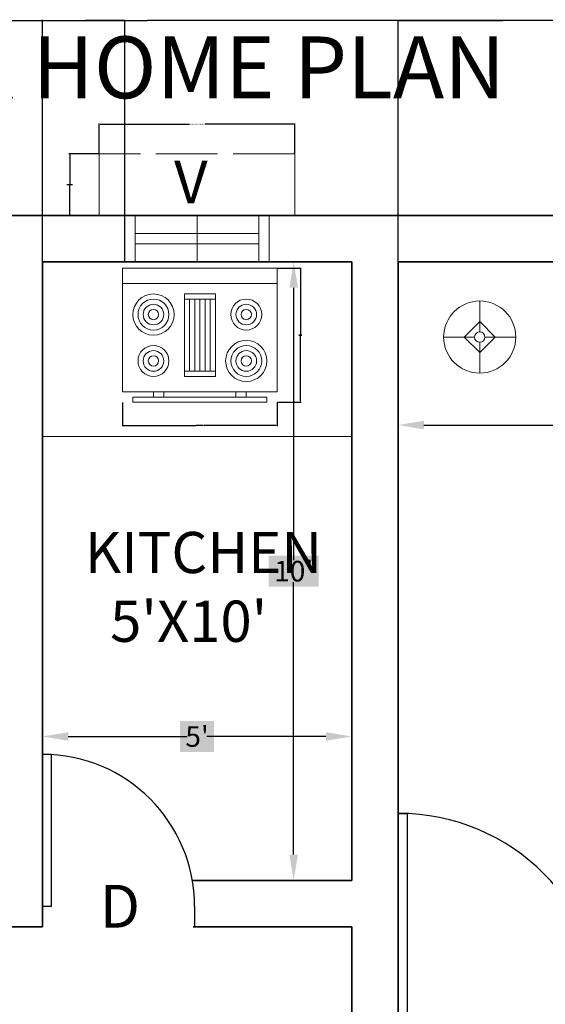
# Model space of a CAD drawing. Units: inches. Extents: x -128 to 854, y -395 to 398.
# Tile 43 of 61: x 107 to 209, y 196 to 387. Entities that reach past the tile are written whole.
import ezdxf

# ---------------------------------------------------------------- set-up
doc = ezdxf.new("R2010")
doc.units = ezdxf.units.IN
doc.header["$MEASUREMENT"] = 0
doc.linetypes.add('ACAD_ISO02W100', pattern=[15, 12, -3])
for name, color, linetype, lineweight in [('A-ANNO-DIMS', 2, 'Continuous', 18), ('A-ANNO-TEXT', 2, 'Continuous', 18), ('A-ANNO-TITL', 7, 'Continuous', 25), ('A-AREA-IDEN', 1, 'Continuous', 18), ('A-DOOR', 4, 'Continuous', 25), ('A-EQPM', 9, 'Continuous', 18), ('A-FLOR-FIXT', 9, 'Continuous', 18), ('A-FURN', 8, 'Continuous', 18), ('A-GLAZ', 220, 'Continuous', 18), ('A-GLAZ-OVHD', 220, 'ACAD_ISO02W100', 13), ('A-WALL', 4, 'Continuous', 35)]:
    doc.layers.add(name, color=color, linetype=linetype, lineweight=lineweight)
doc.styles.get("Standard").update_dxf_attribs({"font": 'arial.ttf'})
doc.dimstyles.get("Standard").update_dxf_attribs({"dimtxt": 0.18, "dimasz": 0.18, "dimexe": 0.18, "dimexo": 0.0625, "dimgap": 0.09, "dimtad": 0, "dimtih": 1, "dimtoh": 1, "dimdec": 1, "dimzin": 0, "dimdsep": 46, "dimlunit": 4, "dimtxsty": 'Standard', "dimcen": 0.09, "dimclrd": 1, "dimclre": 2, "dimclrt": 6, "dimadec": 0, "dimazin": 0, "dimtfac": 1, "dimtdec": 1, "dimtofl": 0, "dimtmove": 0, "dimatfit": 3, "dimfxl": 1, "dimtfill": 2, "dimtfillclr": 3, "dimtolj": 1, "dimtzin": 0, "dimarcsym": 0})

# ---------------------------------------------------------------- blocks, each defined once
blk = doc.blocks.new('*U3')
for p, q in [((0, 0), (0, -6)), ((40, 0), (40, -6))]:
    blk.add_line(p, q)
blk.add_lwpolyline([(0, 0), (0, 40), (1.75, 40), (1.75, 0)], close=True)
blk.add_arc((0, 0), 40, 0, 90)
blk = doc.blocks.new('*U4')
for p, q in [((0, 0), (0, -100)), ((750, 0), (750, -100))]:
    blk.add_line(p, q)
blk.add_lwpolyline([(0, 0), (0, 750), (43.75, 750), (43.75, 0)], close=True)
blk.add_arc((0, 0), 750, 0, 90)
blk = doc.blocks.new('Lamp - Table')
for p, q in [((0, 7), (0, 1)), ((0, 3), (-3, 0)), ((3, 0), (0, 3)), ((-1, 0), (-7, 0)), ((-3, 0), (0, -3)), ((0, -3), (3, 0)), ((1, 0), (7, 0)), ((0, -1), (0, -7))]:
    blk.add_line(p, q)
for radius in [7, 1]:
    blk.add_circle((0, 0), radius)
blk = doc.blocks.new('Range-Oven - 30 in top')
for p, q in [((0, -3), (30, -3)), ((12, -6), (18, -6)), ((13, -20), (13, -6)), ((14, -6), (14, -20)), ((15, -20), (15, -6)), ((16, -6), (16, -20)), ((17, -20), (17, -6)), ((18, -20), (12, -20)), ((6, -24), (6, -25)), ((8, -25), (8, -24)), ((22, -25), (22, -24)), ((24, -24), (24, -25))]:
    blk.add_line(p, q)
for points in [[(0, -24), (0, 0), (30, 0), (30, -24)], [(12, -21), (12, -5), (18, -5), (18, -21)], [(2, -26), (2, -25), (28, -25), (28, -26)]]:
    blk.add_lwpolyline(points, close=True)
for centre, radius in [((6, -9), 4), ((6, -9), 3), ((6, -9), 2), ((24, -9), 3), ((24, -9), 2), ((6, -9), 1), ((24, -9), 1), ((6, -18), 3), ((24, -18), 4), ((24, -18), 3), ((6, -18), 2), ((6, -18), 1), ((24, -18), 2), ((24, -18), 1)]:
    blk.add_circle(centre, radius)
blk = doc.blocks.new('*D50')
at = {"layer": 'A-ANNO-DIMS', "color": 0, "lineweight": -2, "transparency": 16777216}
for p, q in [((111.87, 214.74), (111.87, 247.84)), ((116.87, 247.66), (139.94, 247.66)), ((166.87, 247.66), (143.8, 247.66)), ((171.87, 219.8), (171.87, 247.84))]:
    blk.add_line(p, q, dxfattribs=at)
at = {"layer": 'A-ANNO-DIMS', "color": 0, "transparency": 16777216}
for points in [[(116.87, 248.49), (116.87, 246.83), (111.87, 247.66)], [(166.87, 248.49), (166.87, 246.83), (171.87, 247.66)]]:
    blk.add_solid(points, dxfattribs=at)
at = {"layer": 'Defpoints', "color": 0, "transparency": 16777216}
for p in [(111.87, 247.66), (171.87, 219.74), (111.87, 214.68)]:
    blk.add_point(p, dxfattribs=at)
at = {"layer": 'A-ANNO-DIMS', "color": 0, "transparency": 16777216, "insert": (141.87, 247.66), "char_height": 4, "attachment_point": 5, "bg_fill": 1, "box_fill_scale": 1.25, "bg_fill_color": 3, "bg_fill_transparency": 0}
blk.add_mtext("\\A1;5'", dxfattribs=at)
blk = doc.blocks.new('*D51')
at = {"layer": 'A-ANNO-DIMS', "color": 0, "lineweight": -2, "transparency": 16777216}
for p, q in [((171.81, 339.74), (160.43, 339.74)), ((160.61, 334.74), (160.61, 281.87)), ((160.61, 224.74), (160.61, 277.61)), ((171.81, 219.74), (160.43, 219.74))]:
    blk.add_line(p, q, dxfattribs=at)
at = {"layer": 'A-ANNO-DIMS', "color": 0, "transparency": 16777216}
for points in [[(159.78, 334.74), (161.44, 334.74), (160.61, 339.74)], [(159.78, 224.74), (161.44, 224.74), (160.61, 219.74)]]:
    blk.add_solid(points, dxfattribs=at)
at = {"layer": 'Defpoints', "color": 0, "transparency": 16777216}
for p in [(160.61, 339.74), (171.87, 339.74), (171.87, 219.74)]:
    blk.add_point(p, dxfattribs=at)
at = {"layer": 'A-ANNO-DIMS', "color": 0, "transparency": 16777216, "insert": (160.61, 279.74), "char_height": 4, "attachment_point": 5, "bg_fill": 1, "box_fill_scale": 1.25, "bg_fill_color": 3, "bg_fill_transparency": 0}
blk.add_mtext("\\A1;10'", dxfattribs=at)
blk = doc.blocks.new('*D52')
at = {"layer": 'A-ANNO-DIMS', "color": 0, "lineweight": -2, "transparency": 16777216}
for p, q in [((180.87, 339.68), (180.87, 307.9)), ((304.87, 339.68), (304.87, 307.9)), ((185.87, 308.08), (236.1, 308.08)), ((299.87, 308.08), (249.64, 308.08))]:
    blk.add_line(p, q, dxfattribs=at)
at = {"layer": 'A-ANNO-DIMS', "color": 0, "transparency": 16777216}
for points in [[(185.87, 308.91), (185.87, 307.25), (180.87, 308.08)], [(299.87, 308.91), (299.87, 307.25), (304.87, 308.08)]]:
    blk.add_solid(points, dxfattribs=at)
at = {"layer": 'Defpoints', "color": 0, "transparency": 16777216}
for p in [(180.87, 339.74), (304.87, 339.74), (304.87, 308.08)]:
    blk.add_point(p, dxfattribs=at)
at = {"layer": 'A-ANNO-DIMS', "color": 0, "transparency": 16777216, "insert": (242.87, 308.08), "char_height": 4, "attachment_point": 5, "bg_fill": 1, "box_fill_scale": 1.25, "bg_fill_color": 3, "bg_fill_transparency": 0}
blk.add_mtext('\\A1;10\'-4"', dxfattribs=at)
blk = doc.blocks.new('VENT-24IN')
for p, q in [((0, 0), (0, 9)), ((2, 0), (2, 9)), ((14, 0), (14, 9)), ((26, 0), (26, 9)), ((28, 0), (28, 9)), ((2, 5.5), (26, 5.5)), ((2, 3.5), (26, 3.5))]:
    blk.add_line(p, q)
blk = doc.blocks.new('SHADE-24IN')
for p, q in [((0, 0), (0, 12)), ((38, 12), (0, 12)), ((38, 0), (38, 12)), ((5, 0), (0, 0)), ((33, 0), (38, 0))]:
    blk.add_line(p, q)
blk = doc.blocks.new('*D81')
at = {"layer": 'A-ANNO-DIMS', "color": 2, "lineweight": -2, "transparency": 16777216}
for p, q in [((122.87, 360.8), (122.87, 366.62)), ((160.87, 360.8), (160.87, 366.62))]:
    blk.add_line(p, q, dxfattribs=at)
at = {"layer": 'A-ANNO-DIMS', "color": 1, "lineweight": -2, "transparency": 16777216}
for p, q in [((123.05, 366.44), (140.39, 366.44)), ((160.69, 366.44), (143.35, 366.44))]:
    blk.add_line(p, q, dxfattribs=at)
at = {"layer": 'A-ANNO-DIMS', "color": 1, "transparency": 16777216}
for points in [[(123.05, 366.47), (123.05, 366.41), (122.87, 366.44)], [(160.69, 366.47), (160.69, 366.41), (160.87, 366.44)]]:
    blk.add_solid(points, dxfattribs=at)
at = {"layer": 'Defpoints', "color": 0, "transparency": 16777216}
for p in [(160.87, 366.44), (122.87, 360.74), (160.87, 360.74)]:
    blk.add_point(p, dxfattribs=at)
at = {"layer": 'A-ANNO-DIMS', "color": 6, "transparency": 16777216, "insert": (141.87, 366.44), "char_height": 0.18, "attachment_point": 5, "bg_fill": 1, "box_fill_scale": 1.25, "bg_fill_color": 3, "bg_fill_transparency": 0}
blk.add_mtext('\\A1;VENT SHADE 3\'-2" TYP.', dxfattribs=at)
blk = doc.blocks.new('*D82')
at = {"layer": 'A-ANNO-DIMS', "color": 2, "lineweight": -2, "transparency": 16777216}
for p, q in [((122.81, 360.74), (116.99, 360.74)), ((122.81, 348.74), (116.99, 348.74))]:
    blk.add_line(p, q, dxfattribs=at)
at = {"layer": 'A-ANNO-DIMS', "color": 1, "lineweight": -2, "transparency": 16777216}
for p, q in [((117.17, 360.56), (117.17, 354.92)), ((117.17, 348.92), (117.17, 354.56))]:
    blk.add_line(p, q, dxfattribs=at)
at = {"layer": 'A-ANNO-DIMS', "color": 1, "transparency": 16777216}
for points in [[(117.14, 360.56), (117.2, 360.56), (117.17, 360.74)], [(117.14, 348.92), (117.2, 348.92), (117.17, 348.74)]]:
    blk.add_solid(points, dxfattribs=at)
at = {"layer": 'Defpoints', "color": 0, "transparency": 16777216}
for p in [(117.17, 360.74), (122.87, 360.74), (122.87, 348.74)]:
    blk.add_point(p, dxfattribs=at)
at = {"layer": 'A-ANNO-DIMS', "color": 6, "transparency": 16777216, "insert": (117.17, 354.74), "char_height": 0.18, "attachment_point": 5, "bg_fill": 1, "box_fill_scale": 1.25, "bg_fill_color": 3, "bg_fill_transparency": 0}
blk.add_mtext('\\A1;1\'-0" TYP.', dxfattribs=at)
blk = doc.blocks.new('*D95')
at = {"layer": 'A-ANNO-DIMS', "color": 2, "lineweight": -2, "transparency": 16777216}
for p, q in [((127.42, 312.47), (127.42, 307.85)), ((157.42, 312.47), (157.42, 307.85))]:
    blk.add_line(p, q, dxfattribs=at)
at = {"layer": 'A-ANNO-DIMS', "color": 1, "lineweight": -2, "transparency": 16777216}
for p, q in [((127.6, 308.03), (141.61, 308.03)), ((157.24, 308.03), (143.22, 308.03))]:
    blk.add_line(p, q, dxfattribs=at)
at = {"layer": 'A-ANNO-DIMS', "color": 1, "transparency": 16777216}
for points in [[(127.6, 308.06), (127.6, 308), (127.42, 308.03)], [(157.24, 308.06), (157.24, 308), (157.42, 308.03)]]:
    blk.add_solid(points, dxfattribs=at)
at = {"layer": 'Defpoints', "color": 0, "transparency": 16777216}
for p in [(127.42, 312.53), (157.42, 312.53), (157.42, 308.03)]:
    blk.add_point(p, dxfattribs=at)
at = {"layer": 'A-ANNO-DIMS', "color": 6, "transparency": 16777216, "insert": (142.42, 308.03), "char_height": 0.18, "attachment_point": 5, "bg_fill": 1, "box_fill_scale": 1.25, "bg_fill_color": 3, "bg_fill_transparency": 0}
blk.add_mtext('\\A1;RANGE 2\'-6"', dxfattribs=at)
blk = doc.blocks.new('*D96')
at = {"layer": 'A-ANNO-DIMS', "color": 2, "lineweight": -2, "transparency": 16777216}
for p, q in [((157.48, 338.53), (162.1, 338.53)), ((157.48, 312.53), (162.1, 312.53))]:
    blk.add_line(p, q, dxfattribs=at)
at = {"layer": 'A-ANNO-DIMS', "color": 1, "lineweight": -2, "transparency": 16777216}
for p, q in [((161.92, 338.35), (161.92, 325.71)), ((161.92, 312.71), (161.92, 325.35))]:
    blk.add_line(p, q, dxfattribs=at)
at = {"layer": 'A-ANNO-DIMS', "color": 1, "transparency": 16777216}
for points in [[(161.89, 338.35), (161.95, 338.35), (161.92, 338.53)], [(161.89, 312.71), (161.95, 312.71), (161.92, 312.53)]]:
    blk.add_solid(points, dxfattribs=at)
at = {"layer": 'Defpoints', "color": 0, "transparency": 16777216}
for p in [(157.42, 338.53), (161.92, 338.53), (157.42, 312.53)]:
    blk.add_point(p, dxfattribs=at)
at = {"layer": 'A-ANNO-DIMS', "color": 6, "transparency": 16777216, "insert": (161.92, 325.53), "char_height": 0.18, "attachment_point": 5, "bg_fill": 1, "box_fill_scale": 1.25, "bg_fill_color": 3, "bg_fill_transparency": 0}
blk.add_mtext('\\A1;2\'-2"', dxfattribs=at)
blk = doc.blocks.new('*D97')
at = {"layer": 'A-ANNO-DIMS', "color": 2, "lineweight": -2, "transparency": 16777216}
for p, q in [((-50.13, 348.8), (-50.13, 386.74)), ((313.87, 348.8), (313.87, 386.74))]:
    blk.add_line(p, q, dxfattribs=at)
at = {"layer": 'A-ANNO-DIMS', "color": 1, "lineweight": -2, "transparency": 16777216}
for p, q in [((-49.95, 386.56), (131.47, 386.56)), ((313.69, 386.56), (132.27, 386.56))]:
    blk.add_line(p, q, dxfattribs=at)
at = {"layer": 'A-ANNO-DIMS', "color": 1, "transparency": 16777216}
for points in [[(-49.95, 386.59), (-49.95, 386.53), (-50.13, 386.56)], [(313.69, 386.59), (313.69, 386.53), (313.87, 386.56)]]:
    blk.add_solid(points, dxfattribs=at)
at = {"layer": 'Defpoints', "color": 0, "transparency": 16777216}
for p in [(313.87, 386.56), (-50.13, 348.74), (313.87, 348.74)]:
    blk.add_point(p, dxfattribs=at)
at = {"layer": 'A-ANNO-DIMS', "color": 6, "transparency": 16777216, "insert": (131.87, 386.56), "char_height": 0.18, "attachment_point": 5, "bg_fill": 1, "box_fill_scale": 1.25, "bg_fill_color": 3, "bg_fill_transparency": 0}
blk.add_mtext('\\A1;30\'-4"', dxfattribs=at)
blk = doc.blocks.new('*D101')
at = {"layer": 'A-ANNO-DIMS', "color": 2, "lineweight": -2, "transparency": 16777216}
for p, q in [((180.87, 186.8), (180.87, 386.74)), ((220.87, 186.8), (220.87, 386.74))]:
    blk.add_line(p, q, dxfattribs=at)
at = {"layer": 'A-ANNO-DIMS', "color": 1, "lineweight": -2, "transparency": 16777216}
for p, q in [((181.05, 386.56), (200.54, 386.56)), ((220.69, 386.56), (201.2, 386.56))]:
    blk.add_line(p, q, dxfattribs=at)
at = {"layer": 'A-ANNO-DIMS', "color": 1, "transparency": 16777216}
for points in [[(181.05, 386.59), (181.05, 386.53), (180.87, 386.56)], [(220.69, 386.59), (220.69, 386.53), (220.87, 386.56)]]:
    blk.add_solid(points, dxfattribs=at)
at = {"layer": 'Defpoints', "color": 0, "transparency": 16777216}
for p in [(220.87, 386.56), (180.87, 186.74), (220.87, 186.74)]:
    blk.add_point(p, dxfattribs=at)
at = {"layer": 'A-ANNO-DIMS', "color": 6, "transparency": 16777216, "insert": (200.87, 386.56), "char_height": 0.18, "attachment_point": 5, "bg_fill": 1, "box_fill_scale": 1.25, "bg_fill_color": 3, "bg_fill_transparency": 0}
blk.add_mtext('\\A1;3\'-4"', dxfattribs=at)
blk = doc.blocks.new('*D106')
at = {"layer": 'A-ANNO-DIMS', "color": 2, "lineweight": -2, "transparency": 16777216}
for p, q in [((111.87, 339.8), (111.87, 386.74)), ((127.87, 339.8), (127.87, 386.74))]:
    blk.add_line(p, q, dxfattribs=at)
at = {"layer": 'A-ANNO-DIMS', "color": 1, "lineweight": -2, "transparency": 16777216}
for p, q in [((112.05, 386.56), (119.55, 386.56)), ((127.69, 386.56), (120.19, 386.56))]:
    blk.add_line(p, q, dxfattribs=at)
at = {"layer": 'A-ANNO-DIMS', "color": 1, "transparency": 16777216}
for points in [[(112.05, 386.59), (112.05, 386.53), (111.87, 386.56)], [(127.69, 386.59), (127.69, 386.53), (127.87, 386.56)]]:
    blk.add_solid(points, dxfattribs=at)
at = {"layer": 'Defpoints', "color": 0, "transparency": 16777216}
for p in [(127.87, 386.56), (111.87, 339.74), (127.87, 339.74)]:
    blk.add_point(p, dxfattribs=at)
at = {"layer": 'A-ANNO-DIMS', "color": 6, "transparency": 16777216, "insert": (119.87, 386.56), "char_height": 0.18, "attachment_point": 5, "bg_fill": 1, "box_fill_scale": 1.25, "bg_fill_color": 3, "bg_fill_transparency": 0}
blk.add_mtext('\\A1;1\'-4"', dxfattribs=at)

msp = doc.modelspace()

# ---------------------------------------------------------------- linework, layer by layer
at = {"layer": 'A-FLOR-FIXT'}
msp.add_line((111.87, 305.84), (171.87, 305.84), dxfattribs=at)
at = {"layer": 'A-WALL'}
for p, q in [((-50.13, 348.74), (111.87, 348.74)), ((111.87, 348.74), (180.87, 348.74)), ((180.87, 348.74), (313.87, 348.74)), ((111.87, 339.74), (111.87, 210.74)), ((111.87, 339.74), (171.87, 339.74)), ((171.87, 339.74), (171.87, 219.74)), ((171.87, 339.74), (171.87, 219.74)), ((180.87, 339.74), (304.87, 339.74)), ((180.87, 339.74), (180.87, 186.74)), ((171.87, 219.74), (140.96, 219.74)), ((111.87, 210.74), (102.87, 210.74)), ((171.87, 210.74), (141.14, 210.74)), ((171.87, 210.74), (171.87, 186.74))]:
    msp.add_line(p, q, dxfattribs=at)

# ---------------------------------------------------------------- block references
at = {"layer": 'A-DOOR', "xscale": 0.0393700787401575, "yscale": 0.0393700787401575, "zscale": 0.0393700787401575}
msp.add_blockref('*U4', (111.87, 214.68), dxfattribs=at)
at = {"layer": 'A-DOOR'}
msp.add_blockref('*U3', (180.87, 192.74), dxfattribs=at)
at = {"layer": 'A-EQPM'}
msp.add_blockref('Range-Oven - 30 in top', (127.42, 338.53), dxfattribs=at)
at = {"layer": 'A-FURN'}
msp.add_blockref('Lamp - Table', (196.71, 325.16), dxfattribs=at)
at = {"layer": 'A-GLAZ'}
msp.add_blockref('VENT-24IN', (127.87, 339.74), dxfattribs=at)
at = {"layer": 'A-GLAZ-OVHD'}
msp.add_blockref('SHADE-24IN', (122.87, 348.74), dxfattribs=at)

# ---------------------------------------------------------------- texts
at = {"layer": 'A-ANNO-TEXT'}
for s, p in [('V', (137.41, 351.11)), ('D', (123.01, 210.56))]:
    msp.add_text(s, height=8.31, dxfattribs=at).set_placement(p)
at = {"layer": 'A-ANNO-TITL'}
msp.add_text('3BHK HOME PLAN', height=12, dxfattribs=at).set_placement((63.94, 371.49))
at = {"layer": 'A-AREA-IDEN', "insert": (120.12, 287.36), "char_height": 8, "attachment_point": 1}
msp.add_mtext_dynamic_manual_height_columns("KITCHEN\\P  5'X10'", width=99.0352, gutter_width=1, heights=[0], dxfattribs=at)

# ---------------------------------------------------------------- dimensions: what is measured, and where the dimension line sits
at = {"layer": 'A-ANNO-DIMS'}
for base, p1, p2, override, picture, middle in [((313.87, 386.56), (-50.13, 348.74), (313.87, 348.74), {"dimdec": 1, "dimlfac": 1, "dimrnd": 0, "dimzin": 1, "dimdsep": 46, "dimlunit": 4, "dimfrac": 2}, '*D97', (131.87, 386.56)), ((127.87, 386.56), (111.87, 339.74), (127.87, 339.74), {"dimdec": 1, "dimlfac": 1, "dimrnd": 0, "dimzin": 1, "dimdsep": 46, "dimlunit": 4, "dimfrac": 2}, '*D106', (119.87, 386.56)), ((220.87, 386.56), (180.87, 186.74), (220.87, 186.74), {"dimdec": 1, "dimlfac": 1, "dimrnd": 0, "dimzin": 1, "dimdsep": 46, "dimlunit": 4, "dimfrac": 2}, '*D101', (200.87, 386.56)), ((304.87, 308.08), (180.87, 339.74), (304.87, 339.74), {"dimtxt": 4, "dimasz": 5, "dimclrd": 0, "dimclre": 0, "dimclrt": 0}, '*D52', (242.87, 308.08)), ((111.87, 247.66), (171.87, 219.74), (111.87, 214.68), {"dimtxt": 4, "dimasz": 5, "dimclrd": 0, "dimclre": 0, "dimclrt": 0}, '*D50', (141.87, 247.66))]:
    dim = msp.add_linear_dim(base=base, p1=p1, p2=p2, dimstyle='Standard', override=override, dxfattribs=at)
    dim.commit()
    dim.dimension.update_dxf_attribs({"geometry": picture, "text_midpoint": middle})
for base, p1, p2, text, picture, middle in [((160.87, 366.44), (122.87, 360.74), (160.87, 360.74), 'VENT SHADE <> TYP.', '*D81', (141.87, 366.44)), ((157.42, 308.03), (127.42, 312.53), (157.42, 312.53), 'RANGE <>', '*D95', (142.42, 308.03))]:
    dim = msp.add_linear_dim(base=base, p1=p1, p2=p2, text=text, dimstyle='Standard', override={"dimdec": 1, "dimlfac": 1, "dimrnd": 0, "dimzin": 1, "dimdsep": 46, "dimlunit": 4, "dimfrac": 2}, dxfattribs=at)
    dim.commit()
    dim.dimension.update_dxf_attribs({"geometry": picture, "text_midpoint": middle})
dim = msp.add_linear_dim(base=(117.17, 360.74), p1=(122.87, 348.74), p2=(122.87, 360.74), angle=90, text='<> TYP.', dimstyle='Standard', override={"dimdec": 1, "dimlfac": 1, "dimrnd": 0, "dimzin": 1, "dimdsep": 46, "dimlunit": 4, "dimfrac": 2}, dxfattribs=at)
dim.commit()
dim.dimension.update_dxf_attribs({"geometry": '*D82', "text_midpoint": (117.17, 354.74)})
for base, p1, p2, override, picture, middle in [((160.61, 339.74), (171.87, 219.74), (171.87, 339.74), {"dimtxt": 4, "dimasz": 5, "dimclrd": 0, "dimclre": 0, "dimclrt": 0}, '*D51', (160.61, 279.74)), ((161.92, 338.53), (157.42, 312.53), (157.42, 338.53), {"dimdec": 1, "dimlfac": 1, "dimrnd": 0, "dimzin": 1, "dimdsep": 46, "dimlunit": 4, "dimfrac": 2}, '*D96', (161.92, 325.53))]:
    dim = msp.add_linear_dim(base=base, p1=p1, p2=p2, angle=90, dimstyle='Standard', override=override, dxfattribs=at)
    dim.commit()
    dim.dimension.update_dxf_attribs({"geometry": picture, "text_midpoint": middle})

doc.saveas('drawing.dxf')
